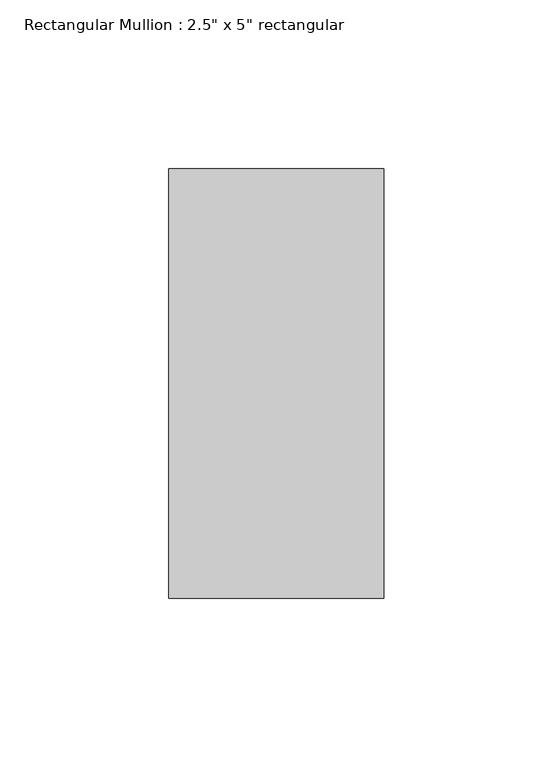
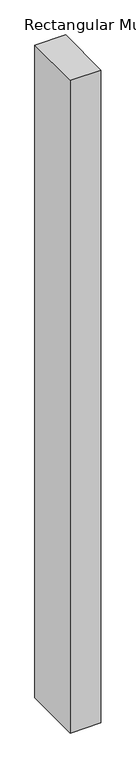
"""IFC4 building model written with IfcOpenShell, lengths in millimetres: member geometry."""

from ifc_helpers import new_model, si_unit, frame, origin, place, context, project, spatial, polyline, outline, extrude, source, transform, mapped, element, save


def member_b1615173(model_context):
    return source(origin(), model_context, "Body", "SweptSolid", [
        extrude(outline(polyline([(0.0, 63.5), (0.0, -63.5), (-63.5, -63.5), (-63.5, 63.5), (0.0, 63.5)])), frame((0.0, 0.0, -1431.017105), z_axis=(0.0, 0.0, 1.0), x_axis=(1.0, 0.0, 0.0)), (0.0, 0.0, 1.0), 1431.017105),
    ])


if __name__ == "__main__":
    model = new_model("IFC4")
    model_context = context("Model", 3, world=origin())
    ifc_project = project(units=[si_unit("LENGTHUNIT", "METRE", prefix="MILLI")], contexts=[model_context])
    site = spatial("IfcSite", under=ifc_project)
    building = spatial("IfcBuilding", under=site)
    placement = place(None, origin())
    member_shape = member_b1615173(model_context)
    element("IfcMember", 1, ObjectType="Rectangular Mullion : 2.5\" x 5\" rectangular", at=placement, inside=building, context=model_context, shape_type="MappedRepresentation", body=[
        mapped(member_shape, transform((0.0, 0.0, 0.0), x_axis=(1.0, 0.0, 0.0), y_axis=(0.0, 1.0, 0.0), z_axis=(0.0, 0.0, 1.0))),
    ])
    save(model, "model.ifc")

# Revit data of these elements
# Type "Rectangular Mullion : 2.5\" x 5\" rectangular"
#   built-in parameter 1007304 = 0.416667 (stored number, unit not read)
#   built-in parameter 1007301 = 0.104167 (stored number, unit not read)
#   built-in parameter 1007300 = 0.104167 (stored number, unit not read)
# Element 1 (IfcMember, "Rectangular Mullion : 2.5\" x 5\" rectangular")
#   Materials on its faces: "Aluminum"
# Materials
#   "Aluminum": class "Metal", colour RGB 247 247 247, transparency 0, Description = "Aluminum 6061", Cost = 0
